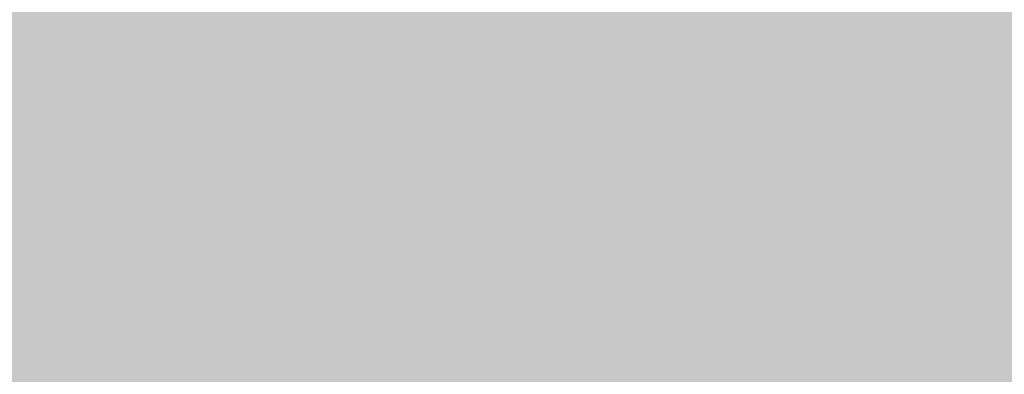
# Model space of a CAD drawing. Units: feet. Extents: x 3168 to 4724, y 827 to 1477.
# Tile 193 of 256: x 3316.07 to 3333.46, y 1087.4 to 1093.65. Entities that reach past the tile are written whole.
import ezdxf

# ---------------------------------------------------------------- set-up
doc = ezdxf.new("R2010")
doc.units = ezdxf.units.FT
doc.layers.add('A-ELEV-PATT', color=8, linetype='Continuous', lineweight=13)

msp = doc.modelspace()

# ---------------------------------------------------------------- hatches: boundary and pattern name
at = {"layer": 'A-ELEV-PATT'}
h = msp.add_hatch(color=256, dxfattribs=at)
h.dxf.hatch_style = 1
edge = h.paths.add_edge_path()
edge.add_ellipse((3552.906, 979.22), major_axis=(36.745, 0), ratio=0.484848, start_angle=0, end_angle=360)
edge = h.paths.add_edge_path()
edge.add_ellipse((3559.892, 929.252), major_axis=(36.745, 0), ratio=0.484848, start_angle=0, end_angle=360)
edge = h.paths.add_edge_path()
edge.add_line((3299.317, 1198.606), (3479.917, 1198.606))
edge.add_line((3479.917, 1198.606), (3479.917, 1209.869))
edge.add_spline(control_points=[(3479.917, 1209.869), (3464.301, 1209.869), (3448.686, 1209.869), (3410.949, 1209.869), (3388.828, 1209.869), (3355.647, 1209.869), (3344.586, 1209.869), (3327.996, 1209.869), (3322.466, 1209.869), (3314.17, 1209.869), (3311.405, 1209.869), (3307.257, 1209.869), (3305.875, 1209.869), (3303.801, 1209.869), (3303.11, 1209.869), (3302.073, 1209.869), (3301.727, 1209.869), (3301.209, 1209.869), (3301.036, 1209.869), (3300.777, 1209.869), (3300.69, 1209.869), (3300.561, 1209.869), (3300.517, 1209.869), (3300.453, 1209.869), (3300.431, 1209.869), (3300.399, 1209.869), (3300.388, 1209.869), (3300.366, 1209.869), (3300.346, 1209.869), (3300.346, 1209.869), (3300.346, 1209.869), (3300.343, 1209.869), (3300.341, 1209.869), (3300.338, 1209.869), (3300.337, 1209.869), (3300.334, 1209.869), (3300.332, 1209.869), (3300.326, 1209.869), (3300.321, 1209.869), (3300.311, 1209.869), (3300.306, 1209.869), (3300.291, 1209.869), (3300.28, 1209.869), (3300.232, 1209.869), (3300.195, 1209.869), (3299.951, 1209.871), (3299.745, 1209.874), (3299.437, 1209.883), (3299.334, 1209.887), (3299.181, 1209.893), (3299.13, 1209.895), (3298.652, 1209.917), (3298.229, 1209.946), (3297.602, 1210.002), (3297.393, 1210.023), (3297.083, 1210.058), (3296.979, 1210.07), (3296.293, 1210.155), (3295.718, 1210.243), (3294.869, 1210.399), (3294.588, 1210.454), (3294.169, 1210.543), (3294.03, 1210.574), (3291.707, 1211.101), (3289.654, 1211.813), (3285.776, 1213.564), (3283.951, 1214.603), (3280.512, 1216.98), (3278.897, 1218.318), (3276.38, 1220.829), (3275.416, 1221.918), (3274.039, 1223.708), (3273.581, 1224.35), (3273.143, 1225.016)], knot_values=[39.119033, 39.119033, 39.119033, 39.119033, 39.286353, 39.286353, 39.523379, 39.523379, 39.641892, 39.641892, 39.701148, 39.701148, 39.730777, 39.730777, 39.745591, 39.745591, 39.752998, 39.752998, 39.756701, 39.756701, 39.758553, 39.758553, 39.759479, 39.759479, 39.759942, 39.759942, 39.760173, 39.760173, 39.760289, 39.760289, 39.760405, 39.760405, 39.760463, 39.760463, 39.763389, 39.763389, 39.764851, 39.764851, 39.767304, 39.767304, 39.773825, 39.773825, 39.78057, 39.78057, 39.79477, 39.79477, 39.845194, 39.845194, 40.126715, 40.126715, 40.267476, 40.267476, 40.337856, 40.337856, 40.927023, 40.927023, 41.221606, 41.221606, 41.368898, 41.368898, 42.202622, 42.202622, 42.619485, 42.619485, 42.827916, 42.827916, 46.118323, 46.118323, 49.408731, 49.408731, 52.699139, 52.699139, 54.927489, 54.927489, 56.104228, 56.104228, 56.104228, 56.104228], weights=[1, 1, 1, 1, 1, 1, 1, 1, 1, 1, 1, 1, 1, 1, 1, 1, 1, 1, 1, 1, 1, 1, 1, 1, 1, 1, 1, 1, 1, 1, 1, 1, 1, 1, 1, 1, 1, 1, 1, 1, 1, 1, 1, 1, 1, 1, 1, 1, 1, 1, 1, 1, 1, 1, 1, 1, 1, 1, 1, 1, 1, 1, 1, 1, 1, 1, 1, 1, 1, 1, 1, 1, 1, 1], degree=3, periodic=0)
edge.add_line((3273.143, 1225.016), (3273.143, 1099.016))
edge.add_line((3273.143, 1099.016), (3299.317, 1099.016))
edge.add_line((3299.317, 1099.016), (3299.317, 1198.606))
edge = h.paths.add_edge_path()
edge.add_line((3304.758, 1324.158), (3479.917, 1324.158))
edge.add_line((3479.917, 1324.158), (3479.917, 1335.715))
edge.add_line((3479.917, 1335.715), (3269.162, 1335.715))
edge.add_spline(control_points=[(3269.162, 1335.715), (3264.024, 1335.715), (3258.364, 1328.958), (3259.264, 1323.9)], knot_values=[0, 0, 0, 0, 15.412191, 15.412191, 15.412191, 15.412191], degree=3, periodic=0)
edge.add_line((3259.264, 1323.9), (3265.517, 1288.769))
edge.add_line((3265.517, 1288.769), (3275.265, 1261.546))
edge.add_line((3275.265, 1261.546), (3304.758, 1261.546))
edge.add_line((3304.758, 1261.546), (3304.758, 1324.158))
h = msp.add_hatch(color=256, dxfattribs=at)
h.dxf.hatch_style = 1
h.paths.add_polyline_path([(3384.525, 1099.016), (3335.029, 1099.016), (3299.317, 1099.016), (3273.143, 1099.016), (3217.565, 1099.016), (3168.069, 827.116), (3335.029, 827.116)])

doc.saveas('drawing.dxf')
